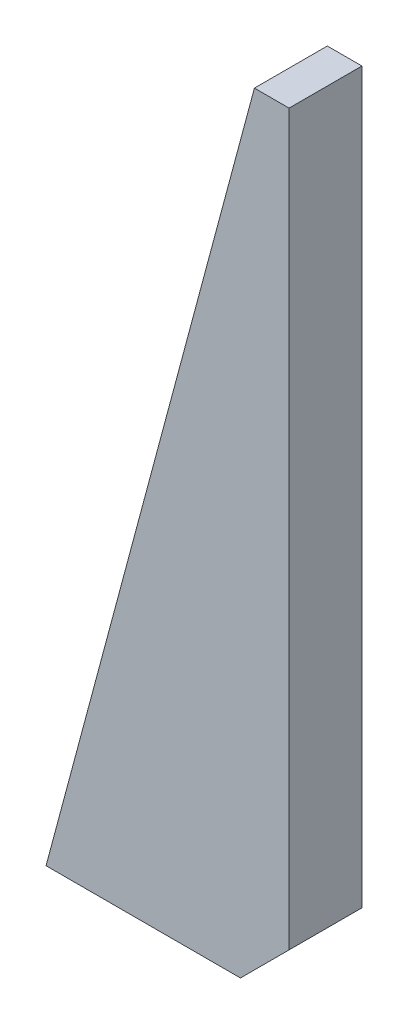
SolidWorks part; units mm, degrees
material "Plain Carbon Steel"
ref_plane "Front Plane" through (0, 0, 0) normal (0, 0, 1) x (1, 0, 0)
ref_plane "Top Plane" through (0, 0, 0) normal (0, 1, 0) x (1, 0, 0)
ref_plane "Right Plane" through (0, 0, 0) normal (1, 0, 0) x (0, 0, -1)
sketch "Gusset Profile Sketch" plane through (0, 0, 0) normal (0, 0, 1) x (1, 0, 0)
  line L0 (0, 0) -> (-50, 0)
  line L1 (-50, 0) -> (-7.1281, 160)
  line L2 (-7.1281, 160) -> (0, 160)
  line L3 (0, 160) -> (0, 0)
  dimension "D1" = 160
  dimension "D2" = 50
  dimension "D3" = 75
extrude "Gusset Plate 15mm" add sketch "Gusset Profile Sketch" along normal blind 15
chamfer "Edge Chamfer 10x45" distance 10 angle 45 1 edges at (0, 0, 7.5)
